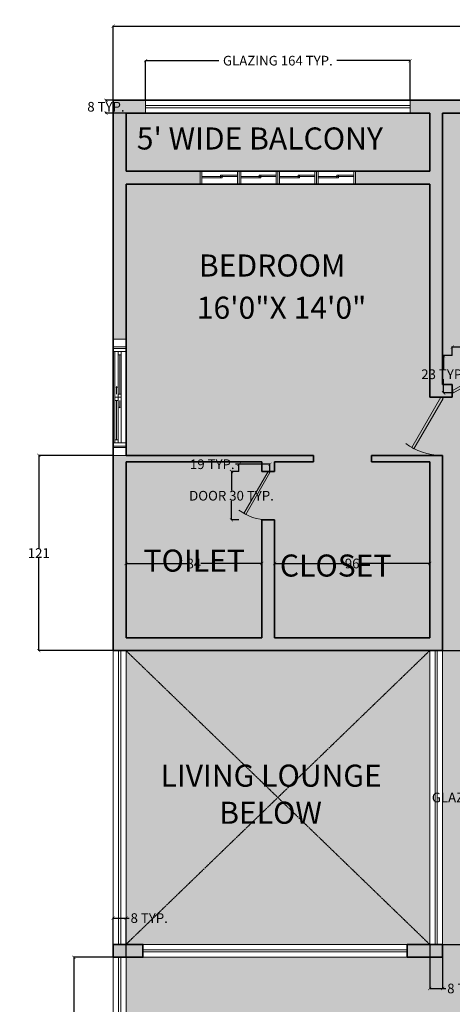
# Model space of a CAD drawing. Units: inches. Extents: x 1704 to 6393, y -157 to 1172.
# Tile 118 of 122: x 4377 to 4645, y 382 to 993. Entities that reach past the tile are written whole.
import ezdxf

# ---------------------------------------------------------------- set-up
doc = ezdxf.new("R2010")
doc.units = ezdxf.units.IN
doc.header["$MEASUREMENT"] = 0
doc.linetypes.add('HIDDEN', pattern=[0.375, 0.25, -0.125])
for name, color, linetype, lineweight in [('A-ANNO-DIMS', 7, 'Continuous', 13), ('A-AREA-IDEN', 7, 'Continuous', 18), ('A-FLOR-OPEN-HIDN', 8, 'HIDDEN', 13), ('A-WALL-PATT', 7, 'Continuous', 13), ('DOORS', 160, 'Continuous', 18), ('GLASS PANEL FASADE', 4, 'Continuous', 18), ('WALLS', 7, 'Continuous', 35), ('WINDOWS', 2, 'Continuous', 18)]:
    doc.layers.add(name, color=color, linetype=linetype, lineweight=lineweight)
doc.layers.add('A-FLOR-PATT', color=7, linetype='Continuous', lineweight=13, true_color=0xf2f2f2)
doc.styles.get("Standard").update_dxf_attribs({"font": 'arial.ttf'})
doc.dimstyles.get("Standard").update_dxf_attribs({"dimtxt": 6, "dimasz": 2, "dimexe": 0.18, "dimexo": 0.0625, "dimgap": 0.09, "dimtad": 0, "dimtih": 1, "dimtoh": 1, "dimdec": 1, "dimzin": 0, "dimdsep": 46, "dimlunit": 3, "dimtxsty": 'Standard', "dimblk": 'ARCHTICK', "dimcen": 0.09, "dimadec": 0, "dimazin": 0, "dimtfac": 1, "dimtdec": 1, "dimtofl": 0, "dimtmove": 0, "dimatfit": 3, "dimfxl": 1, "dimtolj": 1, "dimtzin": 0, "dimarcsym": 0})

# ---------------------------------------------------------------- blocks, each defined once
blk = doc.blocks.new('Door - Left Hung 36 in.')
blk.add_lwpolyline([(0.75, -1.3), (0, 0), (31.18, 18), (31.93, 16.7)], close=True)
blk.add_arc((0, 0), 36, 0, 37.31013)
blk = doc.blocks.new('WIN-SLIDER-72')
for p, q in [((0, 72), (0, 0)), ((0, 72), (8, 72)), ((0, 67.23), (8, 67.23)), ((8, 66.25), (8, 72)), ((1.17, 36), (1.17, 64.3)), ((3.12, 37.95), (3.12, 62.35)), ((4.1, 37.95), (4.1, 62.35)), ((5.07, 37.95), (5.07, 62.35)), ((8, 7.7), (8, 64.3)), ((2.14, 37.95), (2.14, 42.14)), ((1.17, 9.65), (1.17, 34.05)), ((2.14, 9.65), (2.14, 34.05)), ((3.12, 9.65), (3.12, 34.05)), ((4.1, 34.05), (4.1, 29.86)), ((5.07, 36), (5.07, 7.7)), ((0, 4.77), (8, 4.77)), ((8, 5.75), (8, 0)), ((0, 0), (8, 0))]:
    blk.add_line(p, q)
for points in [[(8, 64.3), (8, 66.25), (0, 66.25), (0, 64.3)], [(5.07, 62.35), (5.07, 64.3), (3.12, 64.3), (3.12, 62.35)], [(2.14, 42.65), (1.85, 42.14), (2.44, 42.14)], [(5.07, 36), (5.07, 37.95), (3.12, 37.95), (3.12, 36)], [(3.12, 34.05), (3.12, 36), (1.17, 36), (1.17, 34.05)], [(4.1, 29.35), (3.8, 29.86), (4.39, 29.86)], [(8, 7.7), (8, 5.75), (0, 5.75), (0, 7.7)], [(3.12, 7.7), (3.12, 9.65), (1.17, 9.65), (1.17, 7.7)]]:
    blk.add_lwpolyline(points, close=True)
blk = doc.blocks.new('GLAZ-FOUR-PANEL-96')
for p, q in [((96, 8), (0, 8)), ((0, 8), (0, 0)), ((1, 8), (1, 0)), ((23, 8), (23, 0)), ((24, 8), (24, 0)), ((25, 8), (25, 0)), ((47, 8), (47, 0)), ((48, 8), (48, 0)), ((49, 8), (49, 0)), ((71, 8), (71, 0)), ((72, 8), (72, 0)), ((73, 8), (73, 0)), ((95, 0), (95, 8)), ((96, 0), (96, 8)), ((12.51, 4.77), (1, 4.77)), ((1, 4), (12.51, 4)), ((12.51, 4.77), (12.51, 5.55)), ((12.51, 5.55), (23, 5.55)), ((12.51, 4), (12.51, 4.77)), ((12.51, 4.77), (23, 4.77)), ((12.51, 4), (13.51, 4)), ((13.51, 4), (13.51, 5.55)), ((36.51, 4.77), (25, 4.77)), ((25, 4), (36.51, 4)), ((36.51, 4.77), (36.51, 5.55)), ((36.51, 5.55), (47, 5.55)), ((36.51, 4), (36.51, 4.77)), ((36.51, 4.77), (47, 4.77)), ((36.51, 4), (37.51, 4)), ((37.51, 4), (37.51, 5.55)), ((60.51, 4.77), (49, 4.77)), ((49, 4), (60.51, 4)), ((60.51, 4.77), (60.51, 5.55)), ((60.51, 5.55), (71, 5.55)), ((60.51, 4), (60.51, 4.77)), ((60.51, 4.77), (71, 4.77)), ((60.51, 4), (61.51, 4)), ((61.51, 4), (61.51, 5.55)), ((84.51, 4.77), (73, 4.77)), ((73, 4), (84.51, 4)), ((84.51, 4.77), (84.51, 5.55)), ((84.51, 5.55), (95, 5.55)), ((84.51, 4), (84.51, 4.77)), ((84.51, 4.77), (95, 4.77)), ((84.51, 4), (85.51, 4)), ((85.51, 4), (85.51, 5.55)), ((0, 0), (96, 0))]:
    blk.add_line(p, q)
blk = doc.blocks.new('GLAZ-PANEL-162')
for p, q in [((3.3, 0), (3.3, 162)), ((4.7, 0), (4.7, 162))]:
    blk.add_line(p, q)
blk.add_lwpolyline([(8, 0), (0, 0), (0, 162), (8, 162)], close=True)
blk = doc.blocks.new('GLAZ-PANEL-182')
for p, q in [((3.3, 0), (3.3, 182)), ((4.7, 0), (4.7, 182))]:
    blk.add_line(p, q)
blk.add_lwpolyline([(8, 0), (0, 0), (0, 182), (8, 182)], close=True)
blk = doc.blocks.new('GLAZ-PANEL-164')
for p, q in [((163.71, 4.7), (0, 4.7)), ((163.71, 3.3), (0, 3.3))]:
    blk.add_line(p, q)
blk.add_lwpolyline([(163.71, 8), (163.71, 0), (0, 0), (0, 8)], close=True)
blk = doc.blocks.new('_ArchTick')
at = {"color": 0, "linetype": 'ByBlock', "const_width": 0.15}
blk.add_lwpolyline([(-0.5, -0.5), (0.5, 0.5)], dxfattribs=at)
blk = doc.blocks.new('*D34')
at = {"layer": 'A-ANNO-DIMS', "color": 0, "lineweight": -2, "transparency": 16777216}
for p, q in [((4645.3, 784.51), (4645.3, 790.02)), ((4645.3, 789.84), (4681.3, 789.84)), ((4681.3, 784.51), (4681.3, 790.02)), ((4681.3, 789.84), (4683.3, 789.84))]:
    blk.add_line(p, q, dxfattribs=at)
at = {"layer": 'Defpoints', "color": 0, "lineweight": -3, "transparency": 16777216}
for p in [(4681.3, 789.84), (4645.3, 784.44), (4681.3, 784.44)]:
    blk.add_point(p, dxfattribs=at)
at = {"layer": 'A-ANNO-DIMS', "color": 0, "lineweight": -2, "transparency": 16777216, "xscale": 2, "yscale": 2, "zscale": 2, "rotation": 180}
blk.add_blockref('_ArchTick', (4645.3, 789.84), dxfattribs=at)
at = {"layer": 'A-ANNO-DIMS', "color": 0, "lineweight": -2, "transparency": 16777216, "xscale": 2, "yscale": 2, "zscale": 2}
blk.add_blockref('_ArchTick', (4681.3, 789.84), dxfattribs=at)
at = {"layer": 'A-ANNO-DIMS', "color": 0, "transparency": 16777216, "insert": (4711.58, 789.84), "char_height": 6, "attachment_point": 5}
blk.add_mtext('\\A1;DOOR 36 TYP.', dxfattribs=at)
blk = doc.blocks.new('*D35')
at = {"layer": 'A-ANNO-DIMS', "color": 0, "lineweight": -2, "transparency": 16777216}
for p, q in [((4645.24, 784.44), (4639.72, 784.44)), ((4639.9, 784.44), (4639.9, 776.04)), ((4639.9, 761.32), (4639.9, 769.73)), ((4645.24, 761.32), (4639.72, 761.32))]:
    blk.add_line(p, q, dxfattribs=at)
at = {"layer": 'Defpoints', "color": 0, "lineweight": -3, "transparency": 16777216}
for p in [(4639.9, 784.44), (4645.3, 784.44), (4645.3, 761.32)]:
    blk.add_point(p, dxfattribs=at)
at = {"layer": 'A-ANNO-DIMS', "color": 0, "lineweight": -2, "transparency": 16777216, "xscale": 2, "yscale": 2, "zscale": 2}
for p, rotation in [((4639.9, 784.44), 90), ((4639.9, 761.32), 270)]:
    blk.add_blockref('_ArchTick', p, dxfattribs=dict(at, rotation=rotation))
at = {"layer": 'A-ANNO-DIMS', "color": 0, "transparency": 16777216, "insert": (4639.9, 772.88), "char_height": 6, "attachment_point": 5}
blk.add_mtext('\\A1;23 TYP.', dxfattribs=at)
blk = doc.blocks.new('*D36')
at = {"layer": 'A-ANNO-DIMS', "color": 0, "lineweight": -2, "transparency": 16777216}
for p, q in [((4513.05, 712.62), (4508.44, 712.62)), ((4508.62, 712.62), (4508.62, 700.82)), ((4508.62, 682.62), (4508.62, 694.43)), ((4513.05, 682.62), (4508.44, 682.62))]:
    blk.add_line(p, q, dxfattribs=at)
at = {"layer": 'Defpoints', "color": 0, "lineweight": -3, "transparency": 16777216}
for p in [(4513.12, 712.62), (4508.62, 682.62), (4513.12, 682.62)]:
    blk.add_point(p, dxfattribs=at)
at = {"layer": 'A-ANNO-DIMS', "color": 0, "lineweight": -2, "transparency": 16777216, "xscale": 2, "yscale": 2, "zscale": 2}
for p, rotation in [((4508.62, 712.62), 90), ((4508.62, 682.62), 270)]:
    blk.add_blockref('_ArchTick', p, dxfattribs=dict(at, rotation=rotation))
at = {"layer": 'A-ANNO-DIMS', "color": 0, "transparency": 16777216, "insert": (4508.62, 697.62), "char_height": 6, "attachment_point": 5}
blk.add_mtext('\\A1;DOOR 30 TYP.', dxfattribs=at)
blk = doc.blocks.new('*D37')
at = {"layer": 'A-ANNO-DIMS', "color": 0, "lineweight": -2, "transparency": 16777216}
for p, q in [((4513.12, 717.12), (4511.12, 717.12)), ((4513.12, 712.69), (4513.12, 717.3)), ((4532.38, 717.12), (4513.12, 717.12)), ((4532.38, 712.69), (4532.38, 717.3))]:
    blk.add_line(p, q, dxfattribs=at)
at = {"layer": 'Defpoints', "color": 0, "lineweight": -3, "transparency": 16777216}
for p in [(4513.12, 717.12), (4513.12, 712.62), (4532.38, 712.62)]:
    blk.add_point(p, dxfattribs=at)
at = {"layer": 'A-ANNO-DIMS', "color": 0, "lineweight": -2, "transparency": 16777216, "xscale": 2, "yscale": 2, "zscale": 2, "rotation": 180}
blk.add_blockref('_ArchTick', (4513.12, 717.12), dxfattribs=at)
at = {"layer": 'A-ANNO-DIMS', "color": 0, "lineweight": -2, "transparency": 16777216, "xscale": 2, "yscale": 2, "zscale": 2}
blk.add_blockref('_ArchTick', (4532.38, 717.12), dxfattribs=at)
at = {"layer": 'A-ANNO-DIMS', "color": 0, "transparency": 16777216, "insert": (4496.71, 717.12), "char_height": 6, "attachment_point": 5}
blk.add_mtext('\\A1;19 TYP.', dxfattribs=at)
blk = doc.blocks.new('*D48')
at = {"layer": 'A-ANNO-DIMS', "color": 0, "lineweight": -2, "transparency": 16777216}
for p, q in [((4435.24, 411.62), (4410.82, 411.62)), ((4411, 411.62), (4411, 333.82)), ((4411, 249.62), (4411, 327.43)), ((4435.24, 249.62), (4410.82, 249.62))]:
    blk.add_line(p, q, dxfattribs=at)
at = {"layer": 'Defpoints', "color": 0, "lineweight": -3, "transparency": 16777216}
for p in [(4411, 411.62), (4435.3, 411.62), (4435.3, 249.62)]:
    blk.add_point(p, dxfattribs=at)
at = {"layer": 'A-ANNO-DIMS', "color": 0, "lineweight": -2, "transparency": 16777216, "xscale": 2, "yscale": 2, "zscale": 2}
for p, rotation in [((4411, 411.62), 90), ((4411, 249.62), 270)]:
    blk.add_blockref('_ArchTick', p, dxfattribs=dict(at, rotation=rotation))
at = {"layer": 'A-ANNO-DIMS', "color": 0, "transparency": 16777216, "insert": (4411, 330.62), "char_height": 6, "attachment_point": 5}
blk.add_mtext('\\A1;GLAZING 162 TYP.', dxfattribs=at)
blk = doc.blocks.new('*D49')
at = {"layer": 'A-ANNO-DIMS', "color": 0, "lineweight": -2, "transparency": 16777216}
for p, q in [((4435.3, 411.69), (4435.3, 436.1)), ((4435.3, 435.92), (4443.3, 435.92)), ((4443.3, 411.69), (4443.3, 436.1)), ((4443.3, 435.92), (4445.3, 435.92))]:
    blk.add_line(p, q, dxfattribs=at)
at = {"layer": 'Defpoints', "color": 0, "lineweight": -3, "transparency": 16777216}
for p in [(4443.3, 435.92), (4435.3, 411.62), (4443.3, 411.62)]:
    blk.add_point(p, dxfattribs=at)
at = {"layer": 'A-ANNO-DIMS', "color": 0, "lineweight": -2, "transparency": 16777216, "xscale": 2, "yscale": 2, "zscale": 2, "rotation": 180}
blk.add_blockref('_ArchTick', (4435.3, 435.92), dxfattribs=at)
at = {"layer": 'A-ANNO-DIMS', "color": 0, "lineweight": -2, "transparency": 16777216, "xscale": 2, "yscale": 2, "zscale": 2}
blk.add_blockref('_ArchTick', (4443.3, 435.92), dxfattribs=at)
at = {"layer": 'A-ANNO-DIMS', "color": 0, "transparency": 16777216, "insert": (4457.67, 435.92), "char_height": 6, "attachment_point": 5}
blk.add_mtext('\\A1;8 TYP.', dxfattribs=at)
blk = doc.blocks.new('*D50')
at = {"layer": 'A-ANNO-DIMS', "color": 0, "lineweight": -2, "transparency": 16777216}
for p, q in [((4455.45, 942.69), (4455.45, 967.36)), ((4455.45, 967.18), (4500.76, 967.18)), ((4619.15, 967.18), (4573.84, 967.18)), ((4619.15, 942.69), (4619.15, 967.36))]:
    blk.add_line(p, q, dxfattribs=at)
at = {"layer": 'Defpoints', "color": 0, "lineweight": -3, "transparency": 16777216}
for p in [(4619.15, 967.18), (4455.45, 942.62), (4619.15, 942.62)]:
    blk.add_point(p, dxfattribs=at)
at = {"layer": 'A-ANNO-DIMS', "color": 0, "lineweight": -2, "transparency": 16777216, "xscale": 2, "yscale": 2, "zscale": 2, "rotation": 180}
blk.add_blockref('_ArchTick', (4455.45, 967.18), dxfattribs=at)
at = {"layer": 'A-ANNO-DIMS', "color": 0, "lineweight": -2, "transparency": 16777216, "xscale": 2, "yscale": 2, "zscale": 2}
blk.add_blockref('_ArchTick', (4619.15, 967.18), dxfattribs=at)
at = {"layer": 'A-ANNO-DIMS', "color": 0, "transparency": 16777216, "insert": (4537.3, 967.18), "char_height": 6, "attachment_point": 5}
blk.add_mtext('\\A1;GLAZING 164 TYP.', dxfattribs=at)
blk = doc.blocks.new('*D51')
at = {"layer": 'A-ANNO-DIMS', "color": 0, "lineweight": -2, "transparency": 16777216}
for p, q in [((4455.38, 942.62), (4430.71, 942.62)), ((4430.89, 942.62), (4430.89, 941.78)), ((4455.38, 934.62), (4430.71, 934.62)), ((4430.89, 934.62), (4430.89, 935.47))]:
    blk.add_line(p, q, dxfattribs=at)
at = {"layer": 'Defpoints', "color": 0, "lineweight": -3, "transparency": 16777216}
for p in [(4430.89, 942.62), (4455.45, 942.62), (4455.45, 934.62)]:
    blk.add_point(p, dxfattribs=at)
at = {"layer": 'A-ANNO-DIMS', "color": 0, "lineweight": -2, "transparency": 16777216, "xscale": 2, "yscale": 2, "zscale": 2}
for p, rotation in [((4430.89, 942.62), 90), ((4430.89, 934.62), 270)]:
    blk.add_blockref('_ArchTick', p, dxfattribs=dict(at, rotation=rotation))
at = {"layer": 'A-ANNO-DIMS', "color": 0, "transparency": 16777216, "insert": (4430.89, 938.62), "char_height": 6, "attachment_point": 5}
blk.add_mtext('\\A1;8 TYP.', dxfattribs=at)
blk = doc.blocks.new('*D52')
at = {"layer": 'A-ANNO-DIMS', "color": 0, "lineweight": -2, "transparency": 16777216}
for p, q in [((4639.36, 601.62), (4666.78, 601.62)), ((4666.6, 601.62), (4666.6, 513.82)), ((4666.6, 419.62), (4666.6, 507.43)), ((4639.36, 419.62), (4666.78, 419.62))]:
    blk.add_line(p, q, dxfattribs=at)
at = {"layer": 'Defpoints', "color": 0, "lineweight": -3, "transparency": 16777216}
for p in [(4639.3, 601.62), (4666.6, 601.62), (4639.3, 419.62)]:
    blk.add_point(p, dxfattribs=at)
at = {"layer": 'A-ANNO-DIMS', "color": 0, "lineweight": -2, "transparency": 16777216, "xscale": 2, "yscale": 2, "zscale": 2}
for p, rotation in [((4666.6, 601.62), 90), ((4666.6, 419.62), 270)]:
    blk.add_blockref('_ArchTick', p, dxfattribs=dict(at, rotation=rotation))
at = {"layer": 'A-ANNO-DIMS', "color": 0, "transparency": 16777216, "insert": (4666.6, 510.62), "char_height": 6, "attachment_point": 5}
blk.add_mtext('\\A1;GLAZING 182 TYP.', dxfattribs=at)
blk = doc.blocks.new('*D53')
at = {"layer": 'A-ANNO-DIMS', "color": 0, "lineweight": -2, "transparency": 16777216}
for p, q in [((4631.3, 419.56), (4631.3, 392.14)), ((4639.3, 419.56), (4639.3, 392.14)), ((4631.3, 392.32), (4639.3, 392.32)), ((4639.3, 392.32), (4641.3, 392.32))]:
    blk.add_line(p, q, dxfattribs=at)
at = {"layer": 'Defpoints', "color": 0, "lineweight": -3, "transparency": 16777216}
for p in [(4631.3, 419.62), (4639.3, 419.62), (4639.3, 392.32)]:
    blk.add_point(p, dxfattribs=at)
at = {"layer": 'A-ANNO-DIMS', "color": 0, "lineweight": -2, "transparency": 16777216, "xscale": 2, "yscale": 2, "zscale": 2, "rotation": 180}
blk.add_blockref('_ArchTick', (4631.3, 392.32), dxfattribs=at)
at = {"layer": 'A-ANNO-DIMS', "color": 0, "lineweight": -2, "transparency": 16777216, "xscale": 2, "yscale": 2, "zscale": 2}
blk.add_blockref('_ArchTick', (4639.3, 392.32), dxfattribs=at)
at = {"layer": 'A-ANNO-DIMS', "color": 0, "transparency": 16777216, "insert": (4653.67, 392.32), "char_height": 6, "attachment_point": 5}
blk.add_mtext('\\A1;8 TYP.', dxfattribs=at)
blk = doc.blocks.new('*D107')
at = {"layer": 'A-ANNO-DIMS', "color": 0, "lineweight": -2, "transparency": 16777216}
for p, q in [((4435.3, 942.69), (4435.3, 988.8)), ((4435.3, 988.62), (4707.58, 988.62)), ((4993.3, 988.62), (4721.02, 988.62)), ((4993.3, 801.69), (4993.3, 988.8))]:
    blk.add_line(p, q, dxfattribs=at)
at = {"layer": 'Defpoints', "color": 0, "lineweight": -3, "transparency": 16777216}
for p in [(4993.3, 988.62), (4435.3, 942.62), (4993.3, 801.62)]:
    blk.add_point(p, dxfattribs=at)
at = {"layer": 'A-ANNO-DIMS', "color": 0, "lineweight": -2, "transparency": 16777216, "xscale": 2, "yscale": 2, "zscale": 2, "rotation": 180}
blk.add_blockref('_ArchTick', (4435.3, 988.62), dxfattribs=at)
at = {"layer": 'A-ANNO-DIMS', "color": 0, "lineweight": -2, "transparency": 16777216, "xscale": 2, "yscale": 2, "zscale": 2}
blk.add_blockref('_ArchTick', (4993.3, 988.62), dxfattribs=at)
at = {"layer": 'A-ANNO-DIMS', "color": 0, "transparency": 16777216, "insert": (4714.3, 988.62), "char_height": 6, "attachment_point": 5}
blk.add_mtext('\\A1;558', dxfattribs=at)
blk = doc.blocks.new('*D112')
at = {"layer": 'A-ANNO-DIMS', "color": 0, "lineweight": -2, "transparency": 16777216}
for p, q in [((4435.24, 722.62), (4389.12, 722.62)), ((4389.3, 722.62), (4389.3, 665.23)), ((4389.3, 601.62), (4389.3, 659.02)), ((4435.24, 601.62), (4389.12, 601.62))]:
    blk.add_line(p, q, dxfattribs=at)
at = {"layer": 'Defpoints', "color": 0, "lineweight": -3, "transparency": 16777216}
for p in [(4389.3, 722.62), (4435.3, 722.62), (4435.3, 601.62)]:
    blk.add_point(p, dxfattribs=at)
at = {"layer": 'A-ANNO-DIMS', "color": 0, "lineweight": -2, "transparency": 16777216, "xscale": 2, "yscale": 2, "zscale": 2}
for p, rotation in [((4389.3, 722.62), 90), ((4389.3, 601.62), 270)]:
    blk.add_blockref('_ArchTick', p, dxfattribs=dict(at, rotation=rotation))
at = {"layer": 'A-ANNO-DIMS', "color": 0, "transparency": 16777216, "insert": (4389.3, 662.12), "char_height": 6, "attachment_point": 5}
blk.add_mtext('\\A1;121', dxfattribs=at)
blk = doc.blocks.new('*D113')
at = {"layer": 'A-ANNO-DIMS', "color": 0, "lineweight": -2, "transparency": 16777216}
for p, q in [((4443.3, 609.69), (4443.3, 655.8)), ((4443.3, 655.62), (4480.92, 655.62)), ((4527.3, 655.62), (4489.68, 655.62)), ((4527.3, 609.69), (4527.3, 655.8))]:
    blk.add_line(p, q, dxfattribs=at)
at = {"layer": 'Defpoints', "color": 0, "lineweight": -3, "transparency": 16777216}
for p in [(4527.3, 655.62), (4443.3, 609.62), (4527.3, 609.62)]:
    blk.add_point(p, dxfattribs=at)
at = {"layer": 'A-ANNO-DIMS', "color": 0, "lineweight": -2, "transparency": 16777216, "xscale": 2, "yscale": 2, "zscale": 2, "rotation": 180}
blk.add_blockref('_ArchTick', (4443.3, 655.62), dxfattribs=at)
at = {"layer": 'A-ANNO-DIMS', "color": 0, "lineweight": -2, "transparency": 16777216, "xscale": 2, "yscale": 2, "zscale": 2}
blk.add_blockref('_ArchTick', (4527.3, 655.62), dxfattribs=at)
at = {"layer": 'A-ANNO-DIMS', "color": 0, "transparency": 16777216, "insert": (4485.3, 655.62), "char_height": 6, "attachment_point": 5}
blk.add_mtext('\\A1;84', dxfattribs=at)
blk = doc.blocks.new('*D114')
at = {"layer": 'A-ANNO-DIMS', "color": 0, "lineweight": -2, "transparency": 16777216}
for p, q in [((4535.3, 609.69), (4535.3, 655.8)), ((4535.3, 655.62), (4578.91, 655.62)), ((4631.3, 655.62), (4587.69, 655.62)), ((4631.3, 609.69), (4631.3, 655.8))]:
    blk.add_line(p, q, dxfattribs=at)
at = {"layer": 'Defpoints', "color": 0, "lineweight": -3, "transparency": 16777216}
for p in [(4631.3, 655.62), (4535.3, 609.62), (4631.3, 609.62)]:
    blk.add_point(p, dxfattribs=at)
at = {"layer": 'A-ANNO-DIMS', "color": 0, "lineweight": -2, "transparency": 16777216, "xscale": 2, "yscale": 2, "zscale": 2, "rotation": 180}
blk.add_blockref('_ArchTick', (4535.3, 655.62), dxfattribs=at)
at = {"layer": 'A-ANNO-DIMS', "color": 0, "lineweight": -2, "transparency": 16777216, "xscale": 2, "yscale": 2, "zscale": 2}
blk.add_blockref('_ArchTick', (4631.3, 655.62), dxfattribs=at)
at = {"layer": 'A-ANNO-DIMS', "color": 0, "transparency": 16777216, "insert": (4583.3, 655.62), "char_height": 6, "attachment_point": 5}
blk.add_mtext('\\A1;96', dxfattribs=at)

msp = doc.modelspace()

# ---------------------------------------------------------------- hatches: boundary and pattern name
at = {"layer": 'A-FLOR-PATT', "transparency": 33554516}
h = msp.add_hatch(color=256, dxfattribs=at)
h.dxf.hatch_style = 1
h.paths.add_polyline_path([(4859.3, 934.624), (4639.3, 934.624), (4639.3, 766.624), (4645.3, 766.624), (4645.3, 762.624), (4676.477, 780.624), (4677.227, 779.325), (4677.2, 779.309, -0.0929107), (4681.077, 766.624), (4687.3, 766.624), (4859.3, 766.624), (4859.3, 798.624), (4863.3, 798.624), (4863.3, 766.624), (4875.3, 766.624), (4959.3, 766.624), (4959.3, 834.624), (4923.217, 834.624, -0.0999534), (4920.567, 825.5), (4920.585, 825.49), (4920.085, 824.624), (4899.3, 836.624), (4899.3, 834.624), (4863.3, 834.624), (4859.3, 834.624)])
h.paths.add_polyline_path([(4631.3, 890.624), (4443.3, 890.624), (4443.3, 722.624), (4559.3, 722.624), (4559.3, 718.624), (4535.3, 718.624), (4535.3, 712.624), (4531.3, 712.624), (4532.383, 711.999), (4517.396, 686.04, 0.1210664), (4531.3, 682.624), (4535.3, 682.624), (4535.3, 609.624), (4631.3, 609.624), (4631.3, 718.624), (4595.3, 718.624), (4595.3, 722.624), (4631.3, 722.624), (4637.3, 722.624, -0.1140277), (4621.609, 726.711), (4621.593, 726.684), (4620.293, 727.435), (4638.3, 758.624), (4631.3, 758.624)])
h.paths.add_polyline_path([(4531.3, 712.624), (4527.3, 712.624), (4527.3, 718.624), (4443.3, 718.624), (4443.3, 609.624), (4527.3, 609.624), (4527.3, 682.891, -0.0872676), (4517.396, 686.04), (4517.383, 686.018), (4516.3, 686.643)], flags=17)
h.paths.add_polyline_path([(4631.3, 601.624), (4537.3, 510.624), (4631.3, 419.624)], flags=17)
h.paths.add_polyline_path([(4537.3, 510.624), (4443.3, 419.624), (4453.75, 419.624), (4617.46, 419.624), (4631.3, 419.624)], flags=17)
h.paths.add_polyline_path([(4443.3, 601.624), (4443.3, 419.624), (4537.3, 510.624)], flags=17)
h.paths.add_polyline_path([(4631.3, 601.624), (4443.3, 601.624), (4537.3, 510.624)], flags=17)
h.paths.add_polyline_path([(4637.3, 370.694), (4711.3, 370.694), (4715.3, 370.694, 0.1210664), (4731.986, 374.795), (4713.568, 406.694), (4711.3, 406.694), (4711.3, 419.624), (4712.3, 419.624), (4712.3, 613.124), (4720.3, 613.124), (4720.3, 592.624), (4782.3, 592.624), (4782.3, 657.624), (4720.3, 657.624), (4720.3, 637.124), (4712.3, 637.124), (4712.3, 662.624), (4787.3, 662.624), (4787.3, 654.624), (4787.3, 593.624), (4959.3, 593.624), (4959.3, 654.624), (4811.3, 654.624), (4811.3, 662.624), (4813.69, 662.624), (4813.69, 706.624), (4789.69, 706.624), (4789.69, 712.624), (4729.69, 712.624), (4729.69, 714.624), (4729.69, 758.624), (4681.3, 758.624), (4681.3, 762.624, 0.1210664), (4677.2, 779.309), (4645.3, 760.892), (4645.3, 758.624), (4638.3, 758.624), (4639.6, 757.873), (4621.609, 726.711, 0.1140277), (4637.3, 722.624), (4639.3, 722.624), (4639.3, 601.624), (4639.3, 419.624), (4639.3, 411.624), (4617.46, 411.624), (4453.75, 411.624), (4443.3, 411.624), (4443.3, 249.624), (4637.3, 249.624)])
h.paths.add_polyline_path([(4813.69, 758.624), (4790.69, 758.624), (4790.69, 714.624), (4813.69, 714.624)], flags=17)
h.paths.add_polyline_path([(4789.69, 758.624), (4780.69, 758.624), (4780.69, 714.624), (4789.69, 714.624)], flags=17)
h.paths.add_polyline_path([(4779.69, 758.624), (4770.69, 758.624), (4770.69, 714.624), (4779.69, 714.624)], flags=17)
h.paths.add_polyline_path([(4769.69, 758.624), (4760.69, 758.624), (4760.69, 714.624), (4769.69, 714.624)], flags=17)
h.paths.add_polyline_path([(4759.69, 758.624), (4750.69, 758.624), (4750.69, 714.624), (4759.69, 714.624)], flags=17)
h.paths.add_polyline_path([(4749.69, 758.624), (4740.69, 758.624), (4740.69, 714.624), (4749.69, 714.624)], flags=17)
h.paths.add_polyline_path([(4739.69, 758.624), (4730.69, 758.624), (4730.69, 714.624), (4739.69, 714.624)], flags=17)
h.paths.add_polyline_path([(4823.69, 758.624), (4814.69, 758.624), (4814.69, 714.624), (4823.69, 714.624)], flags=17)
h.paths.add_polyline_path([(4833.69, 758.624), (4824.69, 758.624), (4824.69, 714.624), (4833.69, 714.624)], flags=17)
h.paths.add_polyline_path([(4843.69, 758.624), (4834.69, 758.624), (4834.69, 714.624), (4843.69, 714.624)], flags=17)
h.paths.add_polyline_path([(4909.3, 706.624), (4894.69, 706.624), (4894.69, 662.624), (4909.3, 662.624)], flags=17)
h.paths.add_polyline_path([(4883.69, 706.624), (4874.69, 706.624), (4874.69, 662.624), (4883.69, 662.624)], flags=17)
h.paths.add_polyline_path([(4853.69, 706.624), (4844.69, 706.624), (4844.69, 662.624), (4853.69, 662.624)], flags=17)
h.paths.add_polyline_path([(4833.69, 706.624), (4824.69, 706.624), (4824.69, 662.624), (4833.69, 662.624)], flags=17)
h.paths.add_polyline_path([(4823.69, 706.624), (4814.69, 706.624), (4814.69, 662.624), (4823.69, 662.624)], flags=17)
h.paths.add_polyline_path([(4843.69, 706.624), (4834.69, 706.624), (4834.69, 662.624), (4843.69, 662.624)], flags=17)
h.paths.add_polyline_path([(4863.69, 706.624), (4854.69, 706.624), (4854.69, 662.624), (4863.69, 662.624)], flags=17)
h.paths.add_polyline_path([(4873.69, 706.624), (4864.69, 706.624), (4864.69, 662.624), (4873.69, 662.624)], flags=17)
h.paths.add_polyline_path([(4893.69, 706.624), (4884.69, 706.624), (4884.69, 662.624), (4893.69, 662.624)], flags=17)
h.paths.add_polyline_path([(4853.69, 758.624), (4844.69, 758.624), (4844.69, 714.624), (4853.69, 714.624)], flags=17)
h.paths.add_polyline_path([(4873.69, 758.624), (4864.69, 758.624), (4864.69, 714.624), (4873.69, 714.624)], flags=17)
h.paths.add_polyline_path([(4893.69, 758.624), (4884.69, 758.624), (4884.69, 714.624), (4893.69, 714.624)], flags=17)
h.paths.add_polyline_path([(4909.3, 758.624), (4894.69, 758.624), (4894.69, 714.624), (4909.3, 714.624)], flags=17)
h.paths.add_polyline_path([(4863.69, 758.624), (4854.69, 758.624), (4854.69, 714.624), (4863.69, 714.624)], flags=17)
h.paths.add_polyline_path([(4883.69, 758.624), (4874.69, 758.624), (4874.69, 714.624), (4883.69, 714.624)], flags=17)
h.paths.add_polyline_path([(4907.3, 712.624), (4813.69, 712.624), (4813.69, 708.624), (4907.3, 708.624)], flags=17)
at = {"layer": 'A-FLOR-PATT', "transparency": 33554559}
h = msp.add_hatch(color=256, dxfattribs=at)
h.dxf.hatch_style = 1
h.paths.add_polyline_path([(4631.3, 934.624), (4443.3, 934.624), (4443.3, 898.624), (4631.3, 898.624)])
at = {"layer": 'A-FLOR-PATT', "transparency": 33554511}
h = msp.add_hatch(color=256, dxfattribs=at)
h.dxf.hatch_style = 1
h.paths.add_polyline_path([(4860.3, 585.624), (4839.3, 585.624), (4720.3, 585.624), (4720.3, 466.624), (4766.3, 466.624), (4766.3, 462.624), (4720.3, 462.624), (4720.3, 419.624), (4766.3, 419.624), (4766.3, 415.624), (4767.05, 416.923), (4798.2, 398.938, 0.1210664), (4802.3, 415.624), (4802.3, 419.624), (4959.3, 419.624), (4959.3, 423.456), (4959.3, 424.757), (4959.3, 462.49), (4959.3, 463.791), (4959.3, 467.624), (4959.3, 543.32), (4864.3, 543.32), (4864.3, 462.624), (4802.3, 462.624), (4802.3, 466.624), (4860.3, 466.624)], flags=17)
h.paths.add_polyline_path([(4959.3, 411.624), (4802.077, 411.624, -0.0929107), (4798.2, 398.938), (4767.05, 416.923), (4766.3, 415.624), (4766.3, 411.624), (4719.3, 411.624), (4719.3, 406.694), (4711.3, 406.694), (4711.3, 419.624), (4712.3, 419.624), (4712.3, 613.124), (4720.3, 613.124), (4720.3, 592.624), (4782.3, 592.624), (4782.3, 657.624), (4720.3, 657.624), (4720.3, 637.124), (4712.3, 637.124), (4712.3, 662.624), (4787.3, 662.624), (4787.3, 654.624), (4787.3, 593.624), (4959.3, 593.624), (4959.3, 654.624), (4811.3, 654.624), (4811.3, 662.624), (4813.69, 662.624), (4813.69, 706.624), (4789.69, 706.624), (4789.69, 712.624), (4729.69, 712.624), (4729.69, 714.624), (4729.69, 758.624), (4681.3, 758.624), (4681.3, 766.624), (4687.3, 766.624), (4859.3, 766.624), (4859.3, 798.624), (4863.3, 798.624), (4863.3, 766.624), (4875.3, 766.624), (4959.3, 766.624), (4959.3, 834.624), (4923.3, 834.624), (4923.3, 838.624), (4959.3, 838.624), (4959.3, 892.32), (4863.3, 892.32), (4863.3, 838.624), (4899.3, 838.624), (4899.3, 834.624), (4863.3, 834.624), (4859.3, 834.624), (4859.3, 934.624), (4639.3, 934.624), (4639.3, 766.624), (4645.3, 766.624), (4645.3, 758.624), (4631.3, 758.624), (4631.3, 890.624), (4443.3, 890.624), (4443.3, 722.624), (4559.3, 722.624), (4559.3, 718.624), (4535.3, 718.624), (4535.3, 712.624), (4527.3, 712.624), (4527.3, 718.624), (4443.3, 718.624), (4443.3, 609.624), (4527.3, 609.624), (4527.3, 682.624), (4535.3, 682.624), (4535.3, 609.624), (4631.3, 609.624), (4631.3, 718.624), (4595.3, 718.624), (4595.3, 722.624), (4631.3, 722.624), (4639.3, 722.624), (4639.3, 601.624), (4639.3, 419.624), (4639.3, 411.624), (4617.46, 411.624), (4453.75, 411.624), (4443.3, 411.624), (4443.3, 249.624), (4637.3, 249.624), (4637.3, 370.694), (4711.3, 370.694), (4719.3, 370.694), (4719.3, 145.624), (4959.3, 145.624), (4959.3, 265.624)])
h.paths.add_polyline_path([(4645.3, 362.694), (4645.3, 249.624), (4678.295, 306.15)], flags=17)
h.paths.add_polyline_path([(4711.3, 362.694), (4645.3, 362.694), (4678.295, 306.15)], flags=17)
h.paths.add_polyline_path([(4711.3, 362.694), (4678.295, 306.15), (4711.279, 249.624), (4711.3, 249.624)], flags=17)
at = {"layer": 'A-WALL-PATT'}
h = msp.add_hatch(color=256, dxfattribs=at)
h.dxf.hatch_style = 1
h.paths.add_polyline_path([(4967.3, 942.624), (4699.009, 942.624), (4699.009, 934.624), (4859.3, 934.624), (4859.3, 834.624), (4863.3, 834.624), (4899.3, 834.624), (4899.3, 838.624), (4863.3, 838.624), (4863.3, 934.624), (4959.3, 934.624), (4959.3, 901.624), (4959.3, 834.624), (4959.3, 766.624), (4863.3, 766.624), (4863.3, 798.624), (4859.3, 798.624), (4859.3, 766.624), (4687.3, 766.624), (4681.3, 766.624), (4681.3, 758.624), (4909.3, 758.624), (4909.3, 662.624), (4811.3, 662.624), (4811.3, 654.624), (4959.3, 654.624), (4959.3, 593.624), (4787.3, 593.624), (4787.3, 654.624), (4787.3, 662.624), (4712.3, 662.624), (4712.3, 637.124), (4720.3, 637.124), (4720.3, 657.624), (4782.3, 657.624), (4782.3, 592.624), (4720.3, 592.624), (4720.3, 613.124), (4712.3, 613.124), (4712.3, 419.624), (4711.3, 419.624), (4711.3, 406.694), (4719.3, 406.694), (4719.3, 411.624), (4766.3, 411.624), (4766.3, 419.624), (4720.3, 419.624), (4720.3, 462.624), (4766.3, 462.624), (4766.3, 466.624), (4720.3, 466.624), (4720.3, 585.624), (4839.3, 585.624), (4860.3, 585.624), (4860.3, 466.624), (4802.3, 466.624), (4802.3, 462.624), (4864.3, 462.624), (4864.3, 585.624), (4959.3, 585.624), (4959.3, 542.624), (4959.3, 467.624), (4967.3, 467.624), (4967.3, 559.624), (4993.3, 559.624), (4993.3, 567.435), (4991.3, 567.435), (4991.3, 561.624), (4967.3, 561.624), (4967.3, 613.624), (4991.3, 613.624), (4991.3, 605.789), (4993.3, 605.789), (4993.3, 615.624), (4967.3, 615.624), (4967.3, 654.624), (4967.3, 662.624), (4959.3, 662.624), (4913.3, 662.624), (4913.3, 758.624), (4959.3, 758.624), (4959.3, 692.624), (4967.3, 692.624), (4967.3, 759.624), (4993.3, 759.624), (4993.3, 801.624), (4967.3, 801.624)])
h.paths.add_polyline_path([(4967.3, 799.624), (4991.3, 799.624), (4991.3, 763.624), (4967.3, 763.624)], flags=16)
h.paths.add_polyline_path([(4443.3, 718.624), (4527.3, 718.624), (4527.3, 712.624), (4535.3, 712.624), (4535.3, 718.624), (4559.3, 718.624), (4559.3, 722.624), (4443.3, 722.624), (4435.3, 722.624), (4435.3, 601.624), (4443.3, 601.624), (4639.3, 601.624), (4639.3, 722.624), (4631.3, 722.624), (4595.3, 722.624), (4595.3, 718.624), (4631.3, 718.624), (4631.3, 609.624), (4535.3, 609.624), (4535.3, 682.624), (4527.3, 682.624), (4527.3, 609.624), (4443.3, 609.624)])
h.paths.add_polyline_path([(4443.3, 890.624), (4489.3, 890.624), (4489.3, 898.624), (4443.3, 898.624), (4443.3, 934.624), (4455.446, 934.624), (4455.446, 942.624), (4435.3, 942.624), (4435.3, 794.624), (4443.3, 794.624)])
h.paths.add_polyline_path([(4639.3, 934.624), (4651.009, 934.624), (4651.009, 942.624), (4635.3, 942.624), (4619.155, 942.624), (4619.155, 934.624), (4631.3, 934.624), (4631.3, 898.624), (4585.3, 898.624), (4585.3, 890.624), (4631.3, 890.624), (4631.3, 758.624), (4645.3, 758.624), (4645.3, 766.624), (4639.3, 766.624)])
h.paths.add_polyline_path([(4967.3, 265.624), (4967.3, 309.624), (4959.3, 309.624), (4959.3, 265.624), (4959.3, 145.624), (4719.3, 145.624), (4719.3, 370.694), (4711.3, 370.694), (4711.3, 249.624), (4699.3, 249.624), (4651.3, 249.624), (4639.3, 249.624), (4585.307, 249.624), (4585.307, 241.624), (4639.3, 241.624), (4651.3, 241.624), (4699.3, 241.624), (4711.3, 241.624), (4711.3, 137.624), (4719.3, 137.624), (4959.3, 137.624), (4967.3, 137.624)])
h.paths.add_polyline_path([(4489.307, 249.624), (4435.313, 249.624), (4435.313, 241.624), (4489.307, 241.624)])
h.paths.add_polyline_path([(4967.3, 419.624), (4959.3, 419.624), (4802.3, 419.624), (4802.3, 411.624), (4959.3, 411.624), (4959.3, 381.624), (4967.3, 381.624)])
h.paths.add_polyline_path([(4967.3, 381.624), (4959.3, 381.624), (4959.3, 376.851), (4967.3, 376.851)])
h.paths.add_polyline_path([(4967.3, 314.396), (4959.3, 314.396), (4959.3, 309.624), (4967.3, 309.624)], flags=17)
h.paths.add_polyline_path([(4959.3, 838.624), (4923.3, 838.624), (4923.3, 834.624), (4959.3, 834.624)], flags=17)
at = {"layer": 'A-WALL-PATT', "transparency": 33554559}
h = msp.add_hatch(color=256, dxfattribs=at)
h.dxf.hatch_style = 1
h.paths.add_polyline_path([(4453.75, 419.624), (4435.3, 419.624), (4435.3, 411.624), (4453.75, 411.624)])
h.paths.add_polyline_path([(4639.3, 419.624), (4617.46, 419.624), (4617.46, 411.624), (4639.3, 411.624)])

# ---------------------------------------------------------------- linework, layer by layer
at = {"layer": 'A-FLOR-OPEN-HIDN'}
for p, q in [((4443.3, 419.624), (4631.3, 601.624)), ((4443.3, 601.624), (4631.3, 419.624))]:
    msp.add_line(p, q, dxfattribs=at)
at = {"layer": 'WALLS'}
for p, q in [((4967.3, 942.624), (4435.3, 942.624)), ((4435.3, 942.624), (4435.3, 601.624)), ((4967.3, 942.624), (4635.3, 942.624)), ((4631.3, 934.624), (4443.3, 934.624)), ((4443.3, 934.624), (4443.3, 898.624)), ((4631.3, 898.624), (4631.3, 934.624)), ((4859.3, 934.624), (4639.3, 934.624)), ((4639.3, 766.624), (4639.3, 934.624)), ((4631.3, 898.624), (4443.3, 898.624)), ((4631.3, 890.624), (4443.3, 890.624)), ((4443.3, 890.624), (4443.3, 722.624)), ((4631.3, 758.624), (4631.3, 890.624)), ((4645.3, 766.624), (4639.3, 766.624)), ((4645.3, 766.624), (4645.3, 758.624)), ((4645.3, 758.624), (4631.3, 758.624)), ((4559.3, 722.624), (4443.3, 722.624)), ((4559.3, 718.624), (4559.3, 722.624)), ((4631.3, 722.624), (4595.3, 722.624)), ((4595.3, 718.624), (4595.3, 722.624)), ((4631.3, 722.624), (4639.3, 722.624)), ((4639.3, 601.624), (4639.3, 722.624)), ((4443.3, 718.624), (4443.3, 609.624)), ((4527.3, 718.624), (4443.3, 718.624)), ((4527.3, 718.624), (4527.3, 712.624)), ((4535.3, 718.624), (4535.3, 712.624)), ((4559.3, 718.624), (4535.3, 718.624)), ((4631.3, 718.624), (4595.3, 718.624)), ((4631.3, 609.624), (4631.3, 718.624)), ((4527.3, 712.624), (4535.3, 712.624)), ((4527.3, 682.624), (4535.3, 682.624)), ((4527.3, 682.624), (4527.3, 609.624)), ((4535.3, 682.624), (4535.3, 609.624)), ((4527.3, 609.624), (4443.3, 609.624)), ((4631.3, 609.624), (4535.3, 609.624)), ((4639.3, 601.624), (4435.3, 601.624))]:
    msp.add_line(p, q, dxfattribs=at)
for points in [[(4435.3, 419.624), (4453.75, 419.624), (4453.75, 411.624), (4435.3, 411.624)], [(4639.3, 419.624), (4617.46, 419.624), (4617.46, 411.624), (4639.3, 411.624)]]:
    msp.add_lwpolyline(points, close=True, dxfattribs=at)

# ---------------------------------------------------------------- block references
at = {"layer": 'DOORS'}
msp.add_blockref('Door - Left Hung 36 in.', (4645.3, 762.624), dxfattribs=at)
at = {"layer": 'DOORS', "rotation": 90}
for p, xscale, yscale, zscale in [((4638.3, 758.624), -1.00038572807606, 1.00038572807606, 1.00038572807606), ((4531.3, 712.624), -0.8333333333333172, 0.8333333333333172, 0.8333333333333172)]:
    msp.add_blockref('Door - Left Hung 36 in.', p, dxfattribs=dict(at, xscale=xscale, yscale=yscale, zscale=zscale))
at = {"layer": 'GLASS PANEL FASADE'}
for name, p in [('GLAZ-PANEL-164', (4455.445, 934.624)), ('GLAZ-FOUR-PANEL-96', (4489.301, 890.624)), ('GLAZ-PANEL-182', (4435.3, 419.624)), ('GLAZ-PANEL-182', (4631.3, 419.624)), ('GLAZ-PANEL-164', (4453.75, 411.624)), ('GLAZ-PANEL-162', (4435.301, 249.624))]:
    msp.add_blockref(name, p, dxfattribs=at)
at = {"layer": 'WINDOWS'}
msp.add_blockref('WIN-SLIDER-72', (4435.301, 722.624), dxfattribs=at)

# ---------------------------------------------------------------- texts
at = {"layer": 'A-ANNO-DIMS'}
msp.add_text('16\'0"X 14\'0"', height=13.6672, dxfattribs=at).set_placement((4487.106, 807.253))
at = {"layer": 'A-AREA-IDEN'}
for s, p in [("5' WIDE BALCONY", (4449.983, 912.124)), ('BEDROOM', (4488.446, 833.423)), ('TOILET', (4454.166, 650.574)), ('CLOSET', (4538.536, 647.519)), ('LIVING LOUNGE', (4464.672, 517.334)), ('BELOW', (4501.004, 494.357))]:
    msp.add_text(s, height=13.6672, dxfattribs=at).set_placement(p)

# ---------------------------------------------------------------- dimensions: what is measured, and where the dimension line sits
at = {"layer": 'A-ANNO-DIMS'}
for base, p1, p2, picture, middle in [((4993.3, 988.624), (4435.3, 942.624), (4993.3, 801.624), '*D107', (4714.3, 988.624)), ((4527.3, 655.624), (4443.3, 609.624), (4527.3, 609.624), '*D113', (4485.3, 655.624)), ((4631.3, 655.624), (4535.3, 609.624), (4631.3, 609.624), '*D114', (4583.3, 655.624))]:
    dim = msp.add_linear_dim(base=base, p1=p1, p2=p2, dimstyle='Standard', override={"dimdec": 0, "dimlfac": 1, "dimrnd": 0, "dimzin": 0, "dimdsep": 46, "dimlunit": 2}, dxfattribs=at)
    dim.commit()
    dim.dimension.update_dxf_attribs({"geometry": picture, "text_midpoint": middle})
for base, p1, p2, text, picture, middle in [((4619.155, 967.18), (4455.446, 942.624), (4619.155, 942.624), 'GLAZING <> TYP.', '*D50', (4537.3, 967.18)), ((4681.3, 789.844), (4645.3, 784.444), (4681.3, 784.444), 'DOOR <> TYP.', '*D34', (4711.581, 789.844)), ((4443.3, 435.924), (4435.3, 411.624), (4443.3, 411.624), '<> TYP.', '*D49', (4457.667, 435.924)), ((4639.3, 392.324), (4631.3, 419.624), (4639.3, 419.624), '<> TYP.', '*D53', (4653.667, 392.324))]:
    dim = msp.add_linear_dim(base=base, p1=p1, p2=p2, text=text, dimstyle='Standard', override={"dimdec": 0, "dimlfac": 1, "dimrnd": 0, "dimzin": 0, "dimdsep": 46, "dimlunit": 2}, dxfattribs=at)
    dim.commit()
    dim.dimension.update_dxf_attribs({"geometry": picture, "text_midpoint": middle})
for base, p1, p2, angle, text, picture, middle in [((4430.889, 942.624), (4455.446, 934.624), (4455.446, 942.624), 90, '<> TYP.', '*D51', (4430.889, 938.624)), ((4639.9, 784.444), (4645.3, 761.325), (4645.3, 784.444), 90, '<> TYP.', '*D35', (4639.9, 772.884)), ((4513.116, 717.124), (4532.383, 712.624), (4513.116, 712.624), 180, '<> TYP.', '*D37', (4496.706, 717.124)), ((4508.616, 682.624), (4513.116, 712.624), (4513.116, 682.624), 270, 'DOOR <> TYP.', '*D36', (4508.616, 697.624)), ((4666.6, 601.624), (4639.3, 419.624), (4639.3, 601.624), 90, 'GLAZING <> TYP.', '*D52', (4666.6, 510.624)), ((4411, 411.624), (4435.3, 249.624), (4435.3, 411.624), 90, 'GLAZING <> TYP.', '*D48', (4411, 330.624))]:
    dim = msp.add_linear_dim(base=base, p1=p1, p2=p2, angle=angle, text=text, dimstyle='Standard', override={"dimdec": 0, "dimlfac": 1, "dimrnd": 0, "dimzin": 0, "dimdsep": 46, "dimlunit": 2}, dxfattribs=at)
    dim.commit()
    dim.dimension.update_dxf_attribs({"geometry": picture, "text_midpoint": middle})
dim = msp.add_linear_dim(base=(4389.3, 722.624), p1=(4435.3, 601.624), p2=(4435.3, 722.624), angle=90, dimstyle='Standard', override={"dimdec": 0, "dimlfac": 1, "dimrnd": 0, "dimzin": 0, "dimdsep": 46, "dimlunit": 2}, dxfattribs=at)
dim.commit()
dim.dimension.update_dxf_attribs({"geometry": '*D112', "text_midpoint": (4389.3, 662.124)})

doc.saveas('drawing.dxf')
